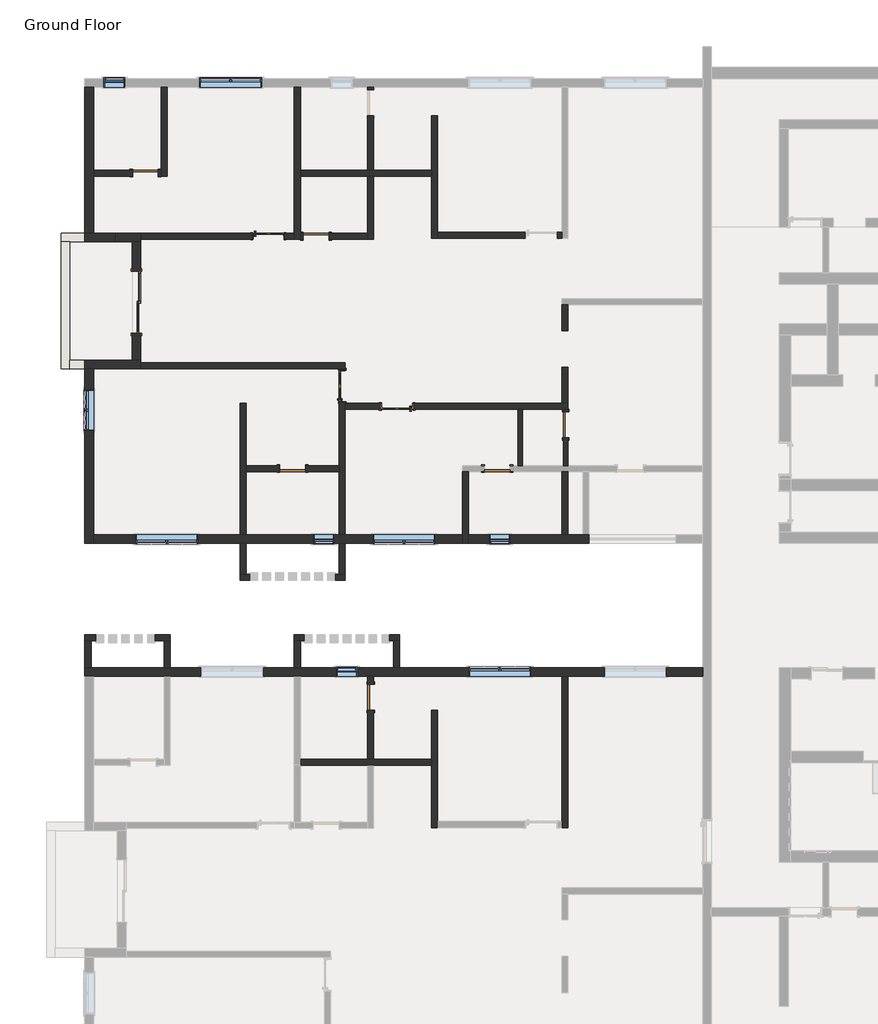
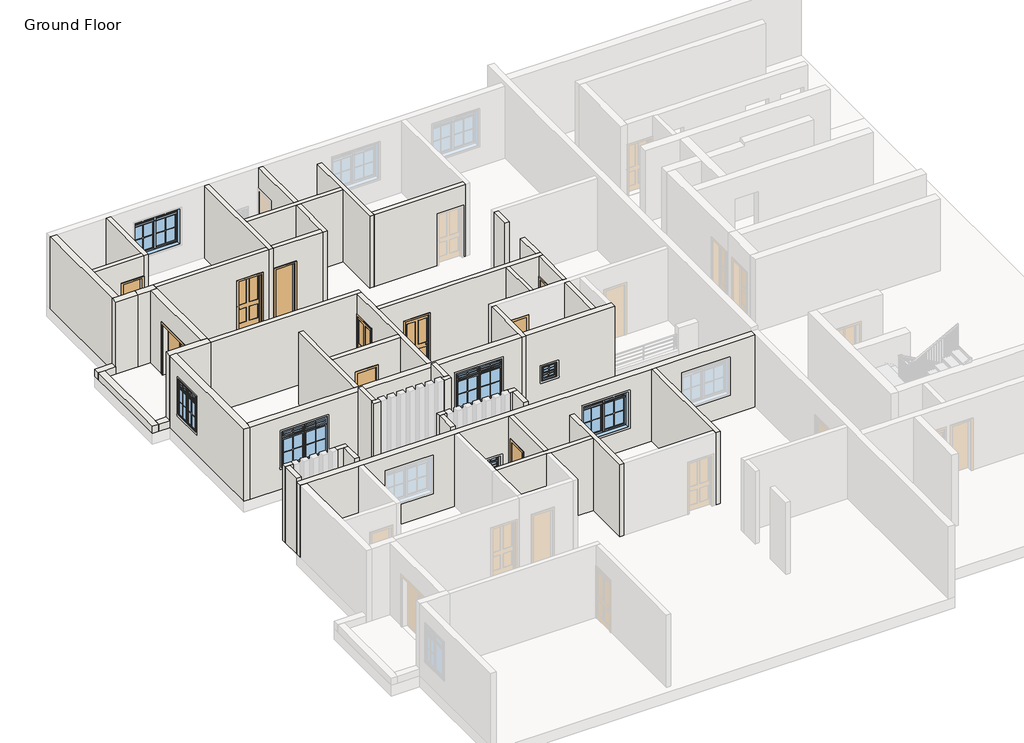
# One storey, part 2 of 9: 49 walls, 10 doors, 9 windows.
"""IFC4 building model written with IfcOpenShell, lengths in millimetres."""

from ifc_helpers import new_model, si_unit, frame, origin, origin_with_axes, place, context, project, spatial, polyline, outline, extrude, faceted_brep, transform, mapped, element, save
from components import door_double_sliding_6_7f701685, door_interior_single_4_panel_wood_3_x_7_bed_room_doors_9f8eaeea, door_0af0cdd0, door_b1104dde, door_6d488673, window_casement_double_awning_double_4_x_5_window_c6f36ef5, window_casement_double_awning_double_6_x_5_2a8633dc, window_double_hung_d0105baa

model = new_model("IFC4")

# Units and contexts
model_context = context("Model", 3, world=origin())
ifc_project = project(units=[si_unit("LENGTHUNIT", "METRE", prefix="MILLI")], contexts=[model_context])

# Site, building, storey
site = spatial("IfcSite", under=ifc_project)
building = spatial("IfcBuilding", under=site)
storey = spatial("IfcBuildingStorey", under=building, Name="Ground Floor", Elevation=0.0)

# Doors
placement = place(None, origin())
door_double_sliding_6_shape = door_double_sliding_6_7f701685(model_context)
element("IfcDoor", 1, ObjectType="Door-Double-Sliding : 6'", at=placement, inside=storey, context=model_context, shape_type="MappedRepresentation", body=[
    mapped(door_double_sliding_6_shape, transform((-13007.9453682, 22386.034892, 0.0), x_axis=(0.0, -1.0, 0.0), y_axis=(1.0, 0.0, 0.0), z_axis=(0.0, 0.0, 1.0))),
])
door_interior_single_4_panel_wood_3_x_7_bed_room_doors_shape = door_interior_single_4_panel_wood_3_x_7_bed_room_doors_9f8eaeea(model_context)
element("IfcDoor", 2, ObjectType="Door-Interior-Single-4_Panel-Wood : 3' x 7' Bed Room Doors", at=placement, inside=storey, context=model_context, shape_type="MappedRepresentation", body=[
    mapped(door_interior_single_4_panel_wood_3_x_7_bed_room_doors_shape, transform((-6826.2203682, 19922.234892, 0.0), x_axis=(0.0, 1.0, 0.0), y_axis=(-1.0, 0.0, 0.0), z_axis=(0.0, 0.0, 1.0))),
])
element("IfcDoor", 3, ObjectType="Door-Interior-Single-4_Panel-Wood : 3' x 7' Bed Room Doors", at=placement, inside=storey, context=model_context, shape_type="MappedRepresentation", body=[
    mapped(door_interior_single_4_panel_wood_3_x_7_bed_room_doors_shape, transform((-5210.1453682, 19322.159892, 0.0), x_axis=(-1.0, 0.0, 0.0), y_axis=(0.0, -1.0, 0.0), z_axis=(0.0, 0.0, 1.0))),
])
element("IfcDoor", 4, ObjectType="Door-Interior-Single-4_Panel-Wood : 3' x 7' Bed Room Doors", at=placement, inside=storey, context=model_context, shape_type="MappedRepresentation", body=[
    mapped(door_interior_single_4_panel_wood_3_x_7_bed_room_doors_shape, transform((-8994.7453682, 24332.309892, 0.0), x_axis=(1.0, 0.0, 0.0), y_axis=(0.0, 1.0, 0.0), z_axis=(0.0, 0.0, 1.0))),
])
door_shape = door_0af0cdd0(model_context)
element("IfcDoor", 5, ObjectType="Single-Flush : 30\" x 80\"", at=placement, inside=storey, context=model_context, shape_type="MappedRepresentation", body=[
    mapped(door_shape, transform((-8283.5453682, 17496.534892, 0.0), x_axis=(-1.0, 0.0, 0.0), y_axis=(0.0, -1.0, 0.0), z_axis=(0.0, 0.0, 1.0))),
])
element("IfcDoor", 6, ObjectType="Single-Flush : 30\" x 80\"", at=placement, inside=storey, context=model_context, shape_type="MappedRepresentation", body=[
    mapped(door_shape, transform((-12614.2453682, 26183.334892, 0.0), x_axis=(1.0, 0.0, 0.0), y_axis=(0.0, 1.0, 0.0), z_axis=(0.0, 0.0, 1.0))),
])
element("IfcDoor", 7, ObjectType="Single-Flush : 30\" x 80\"", at=placement, inside=storey, context=model_context, shape_type="MappedRepresentation", body=[
    mapped(door_shape, transform((-5984.8453682, 10778.234892, 0.0), x_axis=(0.0, 1.0, 0.0), y_axis=(-1.0, 0.0, 0.0), z_axis=(0.0, 0.0, 1.0))),
])
door_2_shape = door_b1104dde(model_context)
element("IfcDoor", 8, ObjectType="Single-Flush : 30\" x 80\"", at=placement, inside=storey, context=model_context, shape_type="MappedRepresentation", body=[
    mapped(door_2_shape, transform((-2263.7453682, 17496.534892, 0.0), x_axis=(1.0, 0.0, 0.0), y_axis=(0.0, 1.0, 0.0), z_axis=(0.0, 0.0, 1.0))),
])
element("IfcDoor", 9, ObjectType="Single-Flush : 30\" x 80\"", at=placement, inside=storey, context=model_context, shape_type="MappedRepresentation", body=[
    mapped(door_2_shape, transform((-7597.7453682, 24329.134892, 0.0), x_axis=(-1.0, 0.0, 0.0), y_axis=(0.0, -1.0, 0.0), z_axis=(0.0, 0.0, 1.0))),
])
door_3_shape = door_6d488673(model_context)
element("IfcDoor", 10, ObjectType="Single-Flush : 30\" x 80\"", at=placement, inside=storey, context=model_context, shape_type="MappedRepresentation", body=[
    mapped(door_3_shape, transform((-250.7953682, 18779.234892, 0.0), x_axis=(0.0, 1.0, 0.0), y_axis=(-1.0, 0.0, 0.0), z_axis=(0.0, 0.0, 1.0))),
])

# Walls
element("IfcWall", 11, at=placement, inside=storey, context=model_context, shape_type="SweptSolid", body=[
    extrude(outline(polyline([(19160.234892, 0.0), (19160.234892, 2133.6), (18398.234892, 2133.6), (18398.234892, 0.0), (17585.434892, 0.0), (17585.434892, 3048.0), (19236.434892, 3048.0), (19236.434892, 0.0), (19160.234892, 0.0)])), frame((-320.6453682, 0.0, 0.0), z_axis=(1.0, 0.0, 0.0), x_axis=(0.0, 1.0, 0.0)), (0.0, 0.0, 1.0), 139.7),
])
element("IfcWall", 12, at=placement, inside=storey, context=model_context, shape_type="SweptSolid", body=[
    extrude(outline(polyline([(-1654.1453682, 17585.434892), (-1654.1453682, 19236.434892), (-1514.4453682, 19236.434892), (-1514.4453682, 17585.434892), (-1654.1453682, 17585.434892)])), origin_with_axes(), (0.0, 0.0, 1.0), 3048.0),
])
element("IfcWall", 13, ObjectType="6\" INTERIOR WALL", at=placement, inside=storey, context=model_context, shape_type="Brep", body=[
    faceted_brep([(-358.7453682, 11387.834892, 0.0), (-358.7453682, 7120.634892, 0.0), (-358.7453682, 6942.834892, 0.0), (-358.7453682, 6942.834892, 3048.0), (-358.7453682, 11387.834892, 3048.0), (-180.9453682, 6942.834892, 0.0), (-180.9453682, 11387.834892, 0.0), (-180.9453682, 11387.834892, 3048.0), (-180.9453682, 6942.834892, 3048.0)], [[[0, 1, 2, 3, 4]], [[5, 6, 7, 8]], [[2, 1, 0, 6, 5]], [[6, 0, 4, 7]], [[2, 5, 8, 3]], [[4, 3, 8, 7]]]),
])
element("IfcWall", 14, ObjectType="6\" INTERIOR WALL", at=placement, inside=storey, context=model_context, shape_type="Brep", body=[
    faceted_brep([(-4194.1453682, 10397.234892, 0.0), (-4194.1453682, 8949.434892, 0.0), (-4194.1453682, 8771.634892, 0.0), (-4194.1453682, 6942.834892, 0.0), (-4194.1453682, 6942.834892, 3048.0), (-4194.1453682, 8771.634892, 3048.0), (-4194.1453682, 8949.434892, 3048.0), (-4194.1453682, 10397.234892, 3048.0), (-4016.3453682, 6942.834892, 0.0), (-4016.3453682, 7120.634892, 0.0), (-4016.3453682, 10397.234892, 0.0), (-4016.3453682, 10397.234892, 3048.0), (-4016.3453682, 7120.634892, 3048.0), (-4016.3453682, 6942.834892, 3048.0)], [[[0, 1, 2, 3, 4, 5, 6, 7]], [[8, 9, 10, 11, 12, 13]], [[3, 2, 1, 0, 10, 9, 8]], [[10, 0, 7, 11]], [[3, 8, 13, 4]], [[7, 6, 5, 4, 13, 12, 11]]]),
])
element("IfcWall", 15, ObjectType="6\" INTERIOR WALL", at=placement, inside=storey, context=model_context, shape_type="SweptSolid", body=[
    extrude(outline(polyline([(11159.234892, 0.0), (11159.234892, 2133.6), (10397.234892, 2133.6), (10397.234892, 0.0), (8949.434892, 0.0), (8949.434892, 3048.0), (11387.834892, 3048.0), (11387.834892, 0.0), (11159.234892, 0.0)])), frame((-6073.7453682, 0.0, 0.0), z_axis=(1.0, 0.0, 0.0), x_axis=(0.0, 1.0, 0.0)), (0.0, 0.0, 1.0), 177.8),
])
element("IfcWall", 16, ObjectType="6\" INTERIOR WALL", at=placement, inside=storey, context=model_context, shape_type="Brep", body=[
    faceted_brep([(-8054.9453682, 8771.634892, 0.0), (-6073.7453682, 8771.634892, 0.0), (-5895.9453682, 8771.634892, 0.0), (-4194.1453682, 8771.634892, 0.0), (-4194.1453682, 8771.634892, 3048.0), (-5895.9453682, 8771.634892, 3048.0), (-6073.7453682, 8771.634892, 3048.0), (-8054.9453682, 8771.634892, 3048.0), (-4194.1453682, 8949.434892, 0.0), (-5895.9453682, 8949.434892, 0.0), (-6073.7453682, 8949.434892, 0.0), (-8054.9453682, 8949.434892, 0.0), (-8054.9453682, 8949.434892, 3048.0), (-6073.7453682, 8949.434892, 3048.0), (-5895.9453682, 8949.434892, 3048.0), (-4194.1453682, 8949.434892, 3048.0)], [[[0, 1, 2, 3, 4, 5, 6, 7]], [[8, 9, 10, 11, 12, 13, 14, 15]], [[3, 2, 1, 0, 11, 10, 9, 8]], [[11, 0, 7, 12]], [[3, 8, 15, 4]], [[7, 6, 5, 4, 15, 14, 13, 12]]]),
])
element("IfcWall", 17, ObjectType="6\" INTERIOR WALL", at=placement, inside=storey, context=model_context, shape_type="SweptSolid", body=[
    extrude(outline(polyline([(-358.7453682, 15553.434892), (-358.7453682, 17407.634892), (-180.9453682, 17407.634892), (-180.9453682, 15553.434892), (-358.7453682, 15553.434892)])), origin_with_axes(), (0.0, 0.0, 1.0), 3048.0),
])
element("IfcWall", 18, ObjectType="6\" INTERIOR WALL", at=placement, inside=storey, context=model_context, shape_type="Brep", body=[
    faceted_brep([(-5692.7453682, 19414.234892, 0.0), (-6734.1453682, 19414.234892, 0.0), (-6734.1453682, 19414.234892, 3048.0), (-358.7453682, 19414.234892, 3048.0), (-180.9453682, 19414.234892, 3048.0), (-180.9453682, 19414.234892, 0.0), (-358.7453682, 19414.234892, 0.0), (-4727.5453682, 19414.234892, 0.0), (-4727.5453682, 19414.234892, 2159.0), (-5692.7453682, 19414.234892, 2159.0), (-6734.1453682, 19236.434892, 0.0), (-5692.7453682, 19236.434892, 0.0), (-5692.7453682, 19236.434892, 2159.0), (-4727.5453682, 19236.434892, 2159.0), (-4727.5453682, 19236.434892, 0.0), (-1654.1453682, 19236.434892, 0.0), (-1514.4453682, 19236.434892, 0.0), (-320.6453682, 19236.434892, 0.0), (-180.9453682, 19236.434892, 0.0), (-180.9453682, 19236.434892, 3048.0), (-320.6453682, 19236.434892, 3048.0), (-1514.4453682, 19236.434892, 3048.0), (-1654.1453682, 19236.434892, 3048.0), (-6734.1453682, 19236.434892, 3048.0)], [[[0, 1, 2, 3, 4, 5, 6, 7, 8, 9]], [[10, 11, 12, 13, 14, 15, 16, 17, 18, 19, 20, 21, 22, 23]], [[5, 18, 17, 16, 15, 14, 7, 6]], [[10, 1, 0, 11]], [[18, 5, 4, 19]], [[1, 10, 23, 2]], [[4, 3, 2, 23, 22, 21, 20, 19]], [[9, 12, 11, 0]], [[12, 9, 8, 13]], [[13, 8, 7, 14]]]),
])
element("IfcWall", 19, ObjectType="6\" INTERIOR WALL", at=placement, inside=storey, context=model_context, shape_type="Brep", body=[
    faceted_brep([(-3279.7453682, 17407.634892, 0.0), (-3279.7453682, 15553.434892, 0.0), (-3279.7453682, 15299.434892, 0.0), (-3279.7453682, 15299.434892, 3048.0), (-3279.7453682, 15553.434892, 3048.0), (-3279.7453682, 17407.634892, 3048.0), (-3101.9453682, 15299.434892, 0.0), (-3101.9453682, 15553.434892, 0.0), (-3101.9453682, 17407.634892, 0.0), (-3101.9453682, 17407.634892, 3048.0), (-3101.9453682, 15299.434892, 3048.0)], [[[0, 1, 2, 3, 4, 5]], [[6, 7, 8, 9, 10]], [[2, 1, 0, 8, 7, 6]], [[8, 0, 5, 9]], [[2, 6, 10, 3]], [[5, 4, 3, 10, 9]]]),
])
element("IfcWall", 20, ObjectType="6\" INTERIOR WALL", at=placement, inside=storey, context=model_context, shape_type="Brep", body=[
    faceted_brep([(-9655.1453682, 15553.434892, 0.0), (-9655.1453682, 17407.634892, 0.0), (-9655.1453682, 17585.434892, 0.0), (-9655.1453682, 19414.234892, 0.0), (-9655.1453682, 19414.234892, 3048.0), (-9655.1453682, 17585.434892, 3048.0), (-9655.1453682, 17407.634892, 3048.0), (-9655.1453682, 15553.434892, 3048.0), (-9832.9453682, 19414.234892, 0.0), (-9832.9453682, 15553.434892, 0.0), (-9832.9453682, 15553.434892, 3048.0), (-9832.9453682, 19414.234892, 3048.0)], [[[0, 1, 2, 3, 4, 5, 6, 7]], [[8, 9, 10, 11]], [[3, 2, 1, 0, 9, 8]], [[3, 8, 11, 4]], [[9, 0, 7, 10]], [[7, 6, 5, 4, 11, 10]]]),
])
element("IfcWall", 21, ObjectType="6\" INTERIOR WALL", at=placement, inside=storey, context=model_context, shape_type="SweptSolid", body=[
    extrude(outline(polyline([(0.0, -8664.5453682), (2133.6, -8664.5453682), (2133.6, -7902.5453682), (0.0, -7902.5453682), (0.0, -6911.9453682), (3048.0, -6911.9453682), (3048.0, -9655.1453682), (0.0, -9655.1453682), (0.0, -8664.5453682)])), frame((0.0, 17407.634892, 0.0), z_axis=(0.0, 1.0, 0.0), x_axis=(0.0, 0.0, 1.0)), (0.0, 0.0, 1.0), 177.8),
])
element("IfcWall", 22, ObjectType="6\" INTERIOR WALL", at=placement, inside=storey, context=model_context, shape_type="Brep", body=[
    faceted_brep([(-6911.9453682, 20430.234892, 0.0), (-6911.9453682, 20404.834892, 0.0), (-6911.9453682, 20404.834892, 2159.0), (-6911.9453682, 19439.634892, 2159.0), (-6911.9453682, 19439.634892, 0.0), (-6911.9453682, 17585.434892, 0.0), (-6911.9453682, 17407.634892, 0.0), (-6911.9453682, 15553.434892, 0.0), (-6911.9453682, 15553.434892, 3048.0), (-6911.9453682, 17407.634892, 3048.0), (-6911.9453682, 17585.434892, 3048.0), (-6911.9453682, 20430.234892, 3048.0), (-6734.1453682, 20404.834892, 0.0), (-6734.1453682, 20430.234892, 0.0), (-6734.1453682, 20430.234892, 3048.0), (-6734.1453682, 19414.234892, 3048.0), (-6734.1453682, 19236.434892, 3048.0), (-6734.1453682, 15553.434892, 3048.0), (-6734.1453682, 15553.434892, 0.0), (-6734.1453682, 19236.434892, 0.0), (-6734.1453682, 19414.234892, 0.0), (-6734.1453682, 19439.634892, 0.0), (-6734.1453682, 19439.634892, 2159.0), (-6734.1453682, 20404.834892, 2159.0)], [[[0, 1, 2, 3, 4, 5, 6, 7, 8, 9, 10, 11]], [[12, 13, 14, 15, 16, 17, 18, 19, 20, 21, 22, 23]], [[18, 7, 6, 5, 4, 21, 20, 19]], [[0, 13, 12, 1]], [[7, 18, 17, 8]], [[13, 0, 11, 14]], [[11, 10, 9, 8, 17, 16, 15, 14]], [[23, 2, 1, 12]], [[2, 23, 22, 3]], [[3, 22, 21, 4]]]),
])
element("IfcWall", 23, ObjectType="6\" INTERIOR WALL", at=placement, inside=storey, context=model_context, shape_type="SweptSolid", body=[
    extrude(outline(polyline([(-358.7453682, 21547.834892), (-358.7453682, 22309.834892), (-180.9453682, 22309.834892), (-180.9453682, 21547.834892), (-358.7453682, 21547.834892)])), origin_with_axes(), (0.0, 0.0, 1.0), 3048.0),
])
element("IfcWall", 24, ObjectType="6\" INTERIOR WALL", at=placement, inside=storey, context=model_context, shape_type="SweptSolid", body=[
    extrude(outline(polyline([(-358.7453682, 19414.234892), (-358.7453682, 20481.034892), (-180.9453682, 20481.034892), (-180.9453682, 19414.234892), (-358.7453682, 19414.234892)])), origin_with_axes(), (0.0, 0.0, 1.0), 3048.0),
])
element("IfcWall", 25, ObjectType="6\" INTERIOR WALL", at=placement, inside=storey, context=model_context, shape_type="Brep", body=[
    faceted_brep([(-4194.1453682, 27872.434892, 0.0), (-4194.1453682, 26272.234892, 0.0), (-4194.1453682, 26094.434892, 0.0), (-4194.1453682, 24265.634892, 0.0), (-4194.1453682, 24265.634892, 3048.0), (-4194.1453682, 26094.434892, 3048.0), (-4194.1453682, 26272.234892, 3048.0), (-4194.1453682, 27872.434892, 3048.0), (-4016.3453682, 24265.634892, 0.0), (-4016.3453682, 24443.434892, 0.0), (-4016.3453682, 27872.434892, 0.0), (-4016.3453682, 27872.434892, 3048.0), (-4016.3453682, 24443.434892, 3048.0), (-4016.3453682, 24265.634892, 3048.0)], [[[0, 1, 2, 3, 4, 5, 6, 7]], [[8, 9, 10, 11, 12, 13]], [[3, 2, 1, 0, 10, 9, 8]], [[10, 0, 7, 11]], [[3, 8, 13, 4]], [[7, 6, 5, 4, 13, 12, 11]]]),
])
element("IfcWall", 26, ObjectType="6\" INTERIOR WALL", at=placement, inside=storey, context=model_context, shape_type="SweptSolid", body=[
    extrude(outline(polyline([(28634.434892, 0.0), (28634.434892, 2133.6), (27872.434892, 2133.6), (27872.434892, 0.0), (26272.234892, 0.0), (26272.234892, 3048.0), (28710.634892, 3048.0), (28710.634892, 0.0), (28634.434892, 0.0)])), frame((-6073.7453682, 0.0, 0.0), z_axis=(1.0, 0.0, 0.0), x_axis=(0.0, 1.0, 0.0)), (0.0, 0.0, 1.0), 177.8),
])
element("IfcWall", 27, ObjectType="6\" INTERIOR WALL", at=placement, inside=storey, context=model_context, shape_type="Brep", body=[
    faceted_brep([(-8054.9453682, 26094.434892, 0.0), (-6073.7453682, 26094.434892, 0.0), (-5895.9453682, 26094.434892, 0.0), (-4194.1453682, 26094.434892, 0.0), (-4194.1453682, 26094.434892, 3048.0), (-5895.9453682, 26094.434892, 3048.0), (-6073.7453682, 26094.434892, 3048.0), (-8054.9453682, 26094.434892, 3048.0), (-4194.1453682, 26272.234892, 0.0), (-5895.9453682, 26272.234892, 0.0), (-6073.7453682, 26272.234892, 0.0), (-8054.9453682, 26272.234892, 0.0), (-8054.9453682, 26272.234892, 3048.0), (-6073.7453682, 26272.234892, 3048.0), (-5895.9453682, 26272.234892, 3048.0), (-4194.1453682, 26272.234892, 3048.0)], [[[0, 1, 2, 3, 4, 5, 6, 7]], [[8, 9, 10, 11, 12, 13, 14, 15]], [[3, 2, 1, 0, 11, 10, 9, 8]], [[3, 8, 15, 4]], [[11, 0, 7, 12]], [[7, 6, 5, 4, 15, 14, 13, 12]]]),
])
element("IfcWall", 28, ObjectType="6\" INTERIOR WALL", at=placement, inside=storey, context=model_context, shape_type="Brep", body=[
    faceted_brep([(-8232.7453682, 28710.634892, 0.0), (-8232.7453682, 24418.034892, 0.0), (-8232.7453682, 24240.234892, 0.0), (-8232.7453682, 24240.234892, 3048.0), (-8232.7453682, 28710.634892, 3048.0), (-8054.9453682, 24240.234892, 0.0), (-8054.9453682, 24418.034892, 0.0), (-8054.9453682, 26094.434892, 0.0), (-8054.9453682, 26272.234892, 0.0), (-8054.9453682, 28710.634892, 0.0), (-8054.9453682, 28710.634892, 3048.0), (-8054.9453682, 26272.234892, 3048.0), (-8054.9453682, 26094.434892, 3048.0), (-8054.9453682, 24418.034892, 3048.0), (-8054.9453682, 24240.234892, 3048.0)], [[[0, 1, 2, 3, 4]], [[5, 6, 7, 8, 9, 10, 11, 12, 13, 14]], [[2, 1, 0, 9, 8, 7, 6, 5]], [[9, 0, 4, 10]], [[2, 5, 14, 3]], [[4, 3, 14, 13, 12, 11, 10]]]),
])
element("IfcWall", 29, ObjectType="6\" INTERIOR WALL", at=placement, inside=storey, context=model_context, shape_type="Brep", body=[
    faceted_brep([(-12157.0453682, 28710.634892, 0.0), (-12157.0453682, 26272.234892, 0.0), (-12157.0453682, 26094.434892, 0.0), (-12157.0453682, 26094.434892, 3048.0), (-12157.0453682, 28710.634892, 3048.0), (-11979.2453682, 26094.434892, 0.0), (-11979.2453682, 28710.634892, 0.0), (-11979.2453682, 28710.634892, 3048.0), (-11979.2453682, 26094.434892, 3048.0)], [[[0, 1, 2, 3, 4]], [[5, 6, 7, 8]], [[2, 1, 0, 6, 5]], [[6, 0, 4, 7]], [[2, 5, 8, 3]], [[4, 3, 8, 7]]]),
])
element("IfcWall", 30, ObjectType="6\" INTERIOR WALL", at=placement, inside=storey, context=model_context, shape_type="SweptSolid", body=[
    extrude(outline(polyline([(2133.6, -12233.2453682), (0.0, -12233.2453682), (0.0, -12157.0453682), (3048.0, -12157.0453682), (3048.0, -14138.2453682), (0.0, -14138.2453682), (0.0, -12995.2453682), (2133.6, -12995.2453682), (2133.6, -12233.2453682)])), frame((0.0, 26094.434892, 0.0), z_axis=(0.0, 1.0, 0.0), x_axis=(0.0, 0.0, 1.0)), (0.0, 0.0, 1.0), 177.8),
])
element("IfcWall", 31, ObjectType="6\" INTERIOR WALL", at=placement, inside=storey, context=model_context, shape_type="Brep", body=[
    faceted_brep([(-6073.7453682, 26094.434892, 0.0), (-6073.7453682, 24418.034892, 0.0), (-6073.7453682, 24240.234892, 0.0), (-6073.7453682, 24240.234892, 3048.0), (-6073.7453682, 26094.434892, 3048.0), (-5895.9453682, 24240.234892, 0.0), (-5895.9453682, 26094.434892, 0.0), (-5895.9453682, 26094.434892, 3048.0), (-5895.9453682, 24240.234892, 3048.0)], [[[0, 1, 2, 3, 4]], [[5, 6, 7, 8]], [[2, 1, 0, 6, 5]], [[6, 0, 4, 7]], [[2, 5, 8, 3]], [[4, 3, 8, 7]]]),
])
element("IfcWall", 32, ObjectType="6\" INTERIOR WALL", at=placement, inside=storey, context=model_context, shape_type="SweptSolid", body=[
    extrude(outline(polyline([(0.0, -7978.7453682), (2133.6, -7978.7453682), (2133.6, -7216.7453682), (0.0, -7216.7453682), (0.0, -6073.7453682), (3048.0, -6073.7453682), (3048.0, -8054.9453682), (0.0, -8054.9453682), (0.0, -7978.7453682)])), frame((0.0, 24240.234892, 0.0), z_axis=(0.0, 1.0, 0.0), x_axis=(0.0, 0.0, 1.0)), (0.0, 0.0, 1.0), 177.8),
])
element("IfcWall", 33, ObjectType="6\" INTERIOR WALL", at=placement, inside=storey, context=model_context, shape_type="SweptSolid", body=[
    extrude(outline(polyline([(0.0, -485.7453682), (0.0, -358.7453682), (3048.0, -358.7453682), (3048.0, -4016.3453682), (0.0, -4016.3453682), (0.0, -1450.9453682), (2159.0, -1450.9453682), (2159.0, -485.7453682), (0.0, -485.7453682)])), frame((0.0, 24265.634892, 0.0), z_axis=(0.0, 1.0, 0.0), x_axis=(0.0, 0.0, 1.0)), (0.0, 0.0, 1.0), 177.8),
])
element("IfcWall", 34, ObjectType="6\" INTERIOR WALL", at=placement, inside=storey, context=model_context, shape_type="Brep", body=[
    faceted_brep([(-12753.9453682, 20430.234892, 0.0), (-6911.9453682, 20430.234892, 0.0), (-6734.1453682, 20430.234892, 0.0), (-6734.1453682, 20430.234892, 3048.0), (-12753.9453682, 20430.234892, 3048.0), (-6734.1453682, 20608.034892, 0.0), (-12753.9453682, 20608.034892, 0.0), (-12753.9453682, 20608.034892, 3048.0), (-6734.1453682, 20608.034892, 3048.0)], [[[0, 1, 2, 3, 4]], [[5, 6, 7, 8]], [[2, 1, 0, 6, 5]], [[6, 0, 4, 7]], [[2, 5, 8, 3]], [[4, 3, 8, 7]]]),
])
element("IfcWall", 35, ObjectType="6\" INTERIOR WALL", at=placement, inside=storey, context=model_context, shape_type="SweptSolid", body=[
    extrude(outline(polyline([(0.0, -8512.1453682), (0.0, -8232.7453682), (3048.0, -8232.7453682), (3048.0, -12753.9453682), (0.0, -12753.9453682), (0.0, -9477.3453682), (2159.0, -9477.3453682), (2159.0, -8512.1453682), (0.0, -8512.1453682)])), frame((0.0, 24240.234892, 0.0), z_axis=(0.0, 1.0, 0.0), x_axis=(0.0, 0.0, 1.0)), (0.0, 0.0, 1.0), 177.8),
])
element("IfcWall", 36, ObjectType="6\" INTERIOR WALL", at=placement, inside=storey, context=model_context, shape_type="SweptSolid", body=[
    extrude(outline(polyline([(-8054.9453682, 12429.234892), (-8054.9453682, 11641.834892), (-8232.7453682, 11641.834892), (-8232.7453682, 12429.234892), (-8054.9453682, 12429.234892)])), origin_with_axes(), (0.0, 0.0, 1.0), 3200.4),
])
element("IfcWall", 37, ObjectType="6\" INTERIOR WALL", at=placement, inside=storey, context=model_context, shape_type="SweptSolid", body=[
    extrude(outline(polyline([(-5133.9453682, 12429.234892), (-5133.9453682, 11641.834892), (-5311.7453682, 11641.834892), (-5311.7453682, 12429.234892), (-5133.9453682, 12429.234892)])), origin_with_axes(), (0.0, 0.0, 1.0), 3200.4),
])
element("IfcWall", 38, ObjectType="6\" INTERIOR WALL", at=placement, inside=storey, context=model_context, shape_type="Brep", body=[
    faceted_brep([(-8232.7453682, 12429.234892, 0.0), (-8054.9453682, 12429.234892, 0.0), (-7940.6453682, 12429.234892, 0.0), (-7940.6453682, 12429.234892, 3200.4), (-8054.9453682, 12429.234892, 3200.4), (-8232.7453682, 12429.234892, 3200.4), (-8232.7453682, 12607.034892, 0.0), (-8232.7453682, 12607.034892, 3200.4), (-7940.6453682, 12607.034892, 3200.4), (-7940.6453682, 12607.034892, 0.0)], [[[0, 1, 2, 3, 4, 5]], [[6, 7, 8, 9]], [[2, 1, 0, 6, 9]], [[3, 2, 9, 8]], [[5, 4, 3, 8, 7]], [[0, 5, 7, 6]]]),
])
element("IfcWall", 39, ObjectType="6\" INTERIOR WALL", at=placement, inside=storey, context=model_context, shape_type="Brep", body=[
    faceted_brep([(-5133.9453682, 12607.034892, 0.0), (-5426.0453682, 12607.034892, 0.0), (-5426.0453682, 12607.034892, 3200.4), (-5133.9453682, 12607.034892, 3200.4), (-5133.9453682, 12429.234892, 0.0), (-5133.9453682, 12429.234892, 3200.4), (-5311.7453682, 12429.234892, 3200.4), (-5426.0453682, 12429.234892, 3200.4), (-5426.0453682, 12429.234892, 0.0), (-5311.7453682, 12429.234892, 0.0)], [[[0, 1, 2, 3]], [[4, 5, 6, 7, 8, 9]], [[1, 0, 4, 9, 8]], [[2, 1, 8, 7]], [[3, 2, 7, 6, 5]], [[0, 3, 5, 4]]]),
])
element("IfcWall", 40, ObjectType="6\" INTERIOR WALL", at=placement, inside=storey, context=model_context, shape_type="Brep", body=[
    faceted_brep([(-14214.4453682, 11641.834892, 0.0), (-14214.4453682, 12429.234892, 0.0), (-14214.4453682, 12429.234892, 3200.4), (-14214.4453682, 11641.834892, 3200.4), (-14392.2453682, 11641.834892, 0.0), (-14392.2453682, 11641.834892, 3048.0), (-14392.2453682, 11641.834892, 3200.4), (-14392.2453682, 12429.234892, 3200.4), (-14392.2453682, 12429.234892, 0.0)], [[[0, 1, 2, 3]], [[4, 5, 6, 7, 8]], [[1, 0, 4, 8]], [[3, 2, 7, 6]], [[2, 1, 8, 7]], [[0, 3, 6, 5, 4]]]),
])
element("IfcWall", 41, ObjectType="6\" INTERIOR WALL", at=placement, inside=storey, context=model_context, shape_type="SweptSolid", body=[
    extrude(outline(polyline([(-11890.3453682, 12429.234892), (-11890.3453682, 11641.834892), (-12068.1453682, 11641.834892), (-12068.1453682, 12429.234892), (-11890.3453682, 12429.234892)])), origin_with_axes(), (0.0, 0.0, 1.0), 3200.4),
])
element("IfcWall", 42, ObjectType="6\" INTERIOR WALL", at=placement, inside=storey, context=model_context, shape_type="Brep", body=[
    faceted_brep([(-14392.2453682, 12429.234892, 0.0), (-14214.4453682, 12429.234892, 0.0), (-14074.7453682, 12429.234892, 0.0), (-14074.7453682, 12429.234892, 3200.4), (-14214.4453682, 12429.234892, 3200.4), (-14392.2453682, 12429.234892, 3200.4), (-14392.2453682, 12607.034892, 0.0), (-14392.2453682, 12607.034892, 3200.4), (-14074.7453682, 12607.034892, 3200.4), (-14074.7453682, 12607.034892, 0.0)], [[[0, 1, 2, 3, 4, 5]], [[6, 7, 8, 9]], [[2, 1, 0, 6, 9]], [[3, 2, 9, 8]], [[5, 4, 3, 8, 7]], [[0, 5, 7, 6]]]),
])
element("IfcWall", 43, ObjectType="6\" INTERIOR WALL", at=placement, inside=storey, context=model_context, shape_type="Brep", body=[
    faceted_brep([(-11890.3453682, 12607.034892, 0.0), (-12322.1453682, 12607.034892, 0.0), (-12322.1453682, 12607.034892, 3200.4), (-11890.3453682, 12607.034892, 3200.4), (-11890.3453682, 12429.234892, 0.0), (-11890.3453682, 12429.234892, 3200.4), (-12068.1453682, 12429.234892, 3200.4), (-12322.1453682, 12429.234892, 3200.4), (-12322.1453682, 12429.234892, 0.0), (-12068.1453682, 12429.234892, 0.0)], [[[0, 1, 2, 3]], [[4, 5, 6, 7, 8, 9]], [[1, 0, 4, 9, 8]], [[2, 1, 8, 7]], [[3, 2, 7, 6, 5]], [[0, 3, 5, 4]]]),
])
element("IfcWall", 44, ObjectType="6\" INTERIOR WALL", at=placement, inside=storey, context=model_context, shape_type="SweptSolid", body=[
    extrude(outline(polyline([(-9832.9453682, 14385.034892), (-9832.9453682, 15299.434892), (-9655.1453682, 15299.434892), (-9655.1453682, 14385.034892), (-9832.9453682, 14385.034892)])), origin_with_axes(), (0.0, 0.0, 1.0), 3200.4),
])
element("IfcWall", 45, ObjectType="6\" INTERIOR WALL", at=placement, inside=storey, context=model_context, shape_type="SweptSolid", body=[
    extrude(outline(polyline([(-6911.9453682, 14385.034892), (-6911.9453682, 15299.434892), (-6734.1453682, 15299.434892), (-6734.1453682, 14385.034892), (-6911.9453682, 14385.034892)])), origin_with_axes(), (0.0, 0.0, 1.0), 3200.4),
])
element("IfcWall", 46, ObjectType="6\" INTERIOR WALL", at=placement, inside=storey, context=model_context, shape_type="Brep", body=[
    faceted_brep([(-9832.9453682, 14207.234892, 0.0), (-9540.8453682, 14207.234892, 0.0), (-9540.8453682, 14207.234892, 3200.4), (-9832.9453682, 14207.234892, 3200.4), (-9832.9453682, 14385.034892, 0.0), (-9832.9453682, 14385.034892, 3200.4), (-9655.1453682, 14385.034892, 3200.4), (-9540.8453682, 14385.034892, 3200.4), (-9540.8453682, 14385.034892, 0.0), (-9655.1453682, 14385.034892, 0.0)], [[[0, 1, 2, 3]], [[4, 5, 6, 7, 8, 9]], [[1, 0, 4, 9, 8]], [[2, 1, 8, 7]], [[3, 2, 7, 6, 5]], [[0, 3, 5, 4]]]),
])
element("IfcWall", 47, ObjectType="6\" INTERIOR WALL", at=placement, inside=storey, context=model_context, shape_type="Brep", body=[
    faceted_brep([(-6734.1453682, 14385.034892, 0.0), (-6911.9453682, 14385.034892, 0.0), (-7026.2453682, 14385.034892, 0.0), (-7026.2453682, 14385.034892, 3200.4), (-6911.9453682, 14385.034892, 3200.4), (-6734.1453682, 14385.034892, 3200.4), (-6734.1453682, 14207.234892, 0.0), (-6734.1453682, 14207.234892, 3200.4), (-7026.2453682, 14207.234892, 3200.4), (-7026.2453682, 14207.234892, 0.0)], [[[0, 1, 2, 3, 4, 5]], [[6, 7, 8, 9]], [[2, 1, 0, 6, 9]], [[3, 2, 9, 8]], [[5, 4, 3, 8, 7]], [[0, 5, 7, 6]]]),
])
element("IfcWall", 48, ObjectType="9\" EXTERIOR WALL", at=placement, inside=storey, context=model_context, shape_type="Brep", body=[
    faceted_brep([(3781.4546318, 11641.834892, 0.0), (-5133.9453682, 11641.834892, 0.0), (-5311.7453682, 11641.834892, 0.0), (-8054.9453682, 11641.834892, 0.0), (-8232.7453682, 11641.834892, 0.0), (-11890.3453682, 11641.834892, 0.0), (-12068.1453682, 11641.834892, 0.0), (-14214.4453682, 11641.834892, 0.0), (-14392.2453682, 11641.834892, 0.0), (-14392.2453682, 11641.834892, 3048.0), (3781.4546318, 11641.834892, 3048.0), (-9147.1453682, 11641.834892, 914.4), (-9147.1453682, 11641.834892, 2438.4), (-10975.9453682, 11641.834892, 2438.4), (-10975.9453682, 11641.834892, 914.4), (-1273.1453682, 11641.834892, 914.4), (-1273.1453682, 11641.834892, 2438.4), (-3101.9453682, 11641.834892, 2438.4), (-3101.9453682, 11641.834892, 914.4), (2714.6546318, 11641.834892, 914.4), (2714.6546318, 11641.834892, 2438.4), (885.8546318, 11641.834892, 2438.4), (885.8546318, 11641.834892, 914.4), (-6988.1453682, 11641.834892, 1524.0), (-6988.1453682, 11641.834892, 914.4), (-6378.5453682, 11641.834892, 914.4), (-6378.5453682, 11641.834892, 1524.0), (-14392.2453682, 11387.834892, 0.0), (-14138.2453682, 11387.834892, 0.0), (-12068.1453682, 11387.834892, 0.0), (-11890.3453682, 11387.834892, 0.0), (-8232.7453682, 11387.834892, 0.0), (-8054.9453682, 11387.834892, 0.0), (-6073.7453682, 11387.834892, 0.0), (-5895.9453682, 11387.834892, 0.0), (-358.7453682, 11387.834892, 0.0), (-180.9453682, 11387.834892, 0.0), (3781.4546318, 11387.834892, 0.0), (3781.4546318, 11387.834892, 3048.0), (-180.9453682, 11387.834892, 3048.0), (-358.7453682, 11387.834892, 3048.0), (-5895.9453682, 11387.834892, 3048.0), (-6073.7453682, 11387.834892, 3048.0), (-8054.9453682, 11387.834892, 3048.0), (-8232.7453682, 11387.834892, 3048.0), (-11890.3453682, 11387.834892, 3048.0), (-12068.1453682, 11387.834892, 3048.0), (-14138.2453682, 11387.834892, 3048.0), (-14392.2453682, 11387.834892, 3048.0), (-9147.1453682, 11387.834892, 2438.4), (-9147.1453682, 11387.834892, 914.4), (-10975.9453682, 11387.834892, 914.4), (-10975.9453682, 11387.834892, 2438.4), (-1273.1453682, 11387.834892, 2438.4), (-1273.1453682, 11387.834892, 914.4), (-3101.9453682, 11387.834892, 914.4), (-3101.9453682, 11387.834892, 2438.4), (2714.6546318, 11387.834892, 2438.4), (2714.6546318, 11387.834892, 914.4), (885.8546318, 11387.834892, 914.4), (885.8546318, 11387.834892, 2438.4), (-6988.1453682, 11387.834892, 914.4), (-6988.1453682, 11387.834892, 1524.0), (-6378.5453682, 11387.834892, 1524.0), (-6378.5453682, 11387.834892, 914.4)], [[[0, 1, 2, 3, 4, 5, 6, 7, 8, 9, 10], [11, 12, 13, 14], [15, 16, 17, 18], [19, 20, 21, 22], [23, 24, 25, 26]], [[27, 28, 29, 30, 31, 32, 33, 34, 35, 36, 37, 38, 39, 40, 41, 42, 43, 44, 45, 46, 47, 48], [49, 50, 51, 52], [53, 54, 55, 56], [57, 58, 59, 60], [61, 62, 63, 64]], [[8, 7, 6, 5, 4, 3, 2, 1, 0, 37, 36, 35, 34, 33, 32, 31, 30, 29, 28, 27]], [[37, 0, 10, 38]], [[8, 27, 48, 9]], [[10, 9, 48, 47, 46, 45, 44, 43, 42, 41, 40, 39, 38]], [[50, 49, 12, 11]], [[51, 50, 11, 14]], [[52, 51, 14, 13]], [[49, 52, 13, 12]], [[54, 53, 16, 15]], [[55, 54, 15, 18]], [[56, 55, 18, 17]], [[53, 56, 17, 16]], [[58, 57, 20, 19]], [[59, 58, 19, 22]], [[60, 59, 22, 21]], [[57, 60, 21, 20]], [[24, 23, 62, 61]], [[25, 24, 61, 64]], [[26, 25, 64, 63]], [[23, 26, 63, 62]]]),
])
element("IfcWall", 49, ObjectType="9\" EXTERIOR WALL", at=placement, inside=storey, context=model_context, shape_type="Brep", body=[
    faceted_brep([(-14138.2453682, 15299.434892, 0.0), (-14138.2453682, 15553.434892, 0.0), (-14138.2453682, 20430.234892, 0.0), (-14138.2453682, 20430.234892, 3048.0), (-14138.2453682, 15553.434892, 3048.0), (-14138.2453682, 15299.434892, 3048.0), (-14138.2453682, 19820.634892, 2438.4), (-14138.2453682, 19820.634892, 914.4), (-14138.2453682, 18601.434892, 914.4), (-14138.2453682, 18601.434892, 2438.4), (-14392.2453682, 20430.234892, 0.0), (-14392.2453682, 15299.434892, 0.0), (-14392.2453682, 15299.434892, 3048.0), (-14392.2453682, 20430.234892, 3048.0), (-14392.2453682, 19820.634892, 914.4), (-14392.2453682, 19820.634892, 2438.4), (-14392.2453682, 18601.434892, 2438.4), (-14392.2453682, 18601.434892, 914.4)], [[[0, 1, 2, 3, 4, 5], [6, 7, 8, 9]], [[10, 11, 12, 13], [14, 15, 16, 17]], [[2, 1, 0, 11, 10]], [[11, 0, 5, 12]], [[2, 10, 13, 3]], [[5, 4, 3, 13, 12]], [[7, 6, 15, 14]], [[8, 7, 14, 17]], [[9, 8, 17, 16]], [[6, 9, 16, 15]]]),
])
element("IfcWall", 50, ObjectType="9\" EXTERIOR WALL", at=placement, inside=storey, context=model_context, shape_type="Brep", body=[
    faceted_brep([(-14138.2453682, 15299.434892, 0.0), (-9832.9453682, 15299.434892, 0.0), (-9655.1453682, 15299.434892, 0.0), (-6911.9453682, 15299.434892, 0.0), (-6734.1453682, 15299.434892, 0.0), (-3279.7453682, 15299.434892, 0.0), (-3279.7453682, 15299.434892, 3048.0), (-14138.2453682, 15299.434892, 3048.0), (-12899.9953682, 15299.434892, 914.4), (-12899.9953682, 15299.434892, 2438.4), (-11071.1953682, 15299.434892, 2438.4), (-11071.1953682, 15299.434892, 914.4), (-5921.3453682, 15299.434892, 914.4), (-5921.3453682, 15299.434892, 2438.4), (-4092.5453682, 15299.434892, 2438.4), (-4092.5453682, 15299.434892, 914.4), (-7064.3453682, 15299.434892, 1524.0), (-7064.3453682, 15299.434892, 914.4), (-7673.9453682, 15299.434892, 914.4), (-7673.9453682, 15299.434892, 1524.0), (-3279.7453682, 15553.434892, 0.0), (-6734.1453682, 15553.434892, 0.0), (-6911.9453682, 15553.434892, 0.0), (-9655.1453682, 15553.434892, 0.0), (-9832.9453682, 15553.434892, 0.0), (-14138.2453682, 15553.434892, 0.0), (-14138.2453682, 15553.434892, 3048.0), (-9832.9453682, 15553.434892, 3048.0), (-9655.1453682, 15553.434892, 3048.0), (-6911.9453682, 15553.434892, 3048.0), (-6734.1453682, 15553.434892, 3048.0), (-3279.7453682, 15553.434892, 3048.0), (-12899.9953682, 15553.434892, 2438.4), (-12899.9953682, 15553.434892, 914.4), (-11071.1953682, 15553.434892, 914.4), (-11071.1953682, 15553.434892, 2438.4), (-5921.3453682, 15553.434892, 2438.4), (-5921.3453682, 15553.434892, 914.4), (-4092.5453682, 15553.434892, 914.4), (-4092.5453682, 15553.434892, 2438.4), (-7064.3453682, 15553.434892, 914.4), (-7064.3453682, 15553.434892, 1524.0), (-7673.9453682, 15553.434892, 1524.0), (-7673.9453682, 15553.434892, 914.4)], [[[0, 1, 2, 3, 4, 5, 6, 7], [8, 9, 10, 11], [12, 13, 14, 15], [16, 17, 18, 19]], [[20, 21, 22, 23, 24, 25, 26, 27, 28, 29, 30, 31], [32, 33, 34, 35], [36, 37, 38, 39], [40, 41, 42, 43]], [[5, 4, 3, 2, 1, 0, 25, 24, 23, 22, 21, 20]], [[25, 0, 7, 26]], [[5, 20, 31, 6]], [[7, 6, 31, 30, 29, 28, 27, 26]], [[33, 32, 9, 8]], [[34, 33, 8, 11]], [[35, 34, 11, 10]], [[32, 35, 10, 9]], [[37, 36, 13, 12]], [[38, 37, 12, 15]], [[39, 38, 15, 14]], [[36, 39, 14, 13]], [[17, 16, 41, 40]], [[18, 17, 40, 43]], [[19, 18, 43, 42]], [[16, 19, 42, 41]]]),
])
element("IfcWall", 51, ObjectType="9\" EXTERIOR WALL", at=placement, inside=storey, context=model_context, shape_type="Brep", body=[
    faceted_brep([(-14392.2453682, 28710.634892, 0.0), (-14392.2453682, 24418.034892, 0.0), (-14392.2453682, 24418.034892, 3048.0), (-14392.2453682, 28710.634892, 3048.0), (-14138.2453682, 24418.034892, 0.0), (-14138.2453682, 26094.434892, 0.0), (-14138.2453682, 26272.234892, 0.0), (-14138.2453682, 28710.634892, 0.0), (-14138.2453682, 28710.634892, 3048.0), (-14138.2453682, 26272.234892, 3048.0), (-14138.2453682, 26094.434892, 3048.0), (-14138.2453682, 24418.034892, 3048.0)], [[[0, 1, 2, 3]], [[4, 5, 6, 7, 8, 9, 10, 11]], [[1, 0, 7, 6, 5, 4]], [[7, 0, 3, 8]], [[1, 4, 11, 2]], [[3, 2, 11, 10, 9, 8]]]),
])
element("IfcWall", 52, ObjectType="9\" EXTERIOR WALL", at=placement, inside=storey, context=model_context, shape_type="SweptSolid", body=[
    extrude(outline(polyline([(-14392.2453682, 20430.234892), (-14836.7453682, 20430.234892), (-14836.7453682, 20684.234892), (-14392.2453682, 20684.234892), (-14392.2453682, 20430.234892)])), origin_with_axes(), (0.0, 0.0, 1.0), 304.8),
])
element("IfcWall", 53, ObjectType="9\" EXTERIOR WALL", at=placement, inside=storey, context=model_context, shape_type="Brep", body=[
    faceted_brep([(-13490.5453682, 24164.034892, 0.0), (-13007.9453682, 24164.034892, 0.0), (-12753.9453682, 24164.034892, 0.0), (-12753.9453682, 24164.034892, 3048.0), (-13007.9453682, 24164.034892, 3048.0), (-13490.5453682, 24164.034892, 3048.0), (-12753.9453682, 24418.034892, 0.0), (-13490.5453682, 24418.034892, 0.0), (-13490.5453682, 24418.034892, 3048.0), (-12753.9453682, 24418.034892, 3048.0), (-12753.9453682, 24240.234892, 0.0), (-12753.9453682, 24240.234892, 3048.0)], [[[0, 1, 2, 3, 4, 5]], [[6, 7, 8, 9]], [[2, 1, 0, 7, 6, 10]], [[7, 0, 5, 8]], [[2, 10, 6, 9, 11, 3]], [[4, 3, 11, 9, 8, 5]]]),
])
element("IfcWall", 54, ObjectType="9\" EXTERIOR WALL", at=placement, inside=storey, context=model_context, shape_type="SweptSolid", body=[
    extrude(outline(polyline([(23300.434892, 0.0), (23300.434892, 2133.6), (21471.634892, 2133.6), (21471.634892, 0.0), (20684.234892, 0.0), (20684.234892, 3048.0), (24164.034892, 3048.0), (24164.034892, 0.0), (23300.434892, 0.0)])), frame((-13007.9453682, 0.0, 0.0), z_axis=(1.0, 0.0, 0.0), x_axis=(0.0, 1.0, 0.0)), (0.0, 0.0, 1.0), 254.0),
])
element("IfcWall", 55, ObjectType="9\" EXTERIOR WALL", at=placement, inside=storey, context=model_context, shape_type="Brep", body=[
    faceted_brep([(-13490.5453682, 24418.034892, 0.0), (-14138.2453682, 24418.034892, 0.0), (-14392.2453682, 24418.034892, 0.0), (-14392.2453682, 24418.034892, 304.8), (-14392.2453682, 24418.034892, 3048.0), (-14138.2453682, 24418.034892, 3048.0), (-13490.5453682, 24418.034892, 3048.0), (-14392.2453682, 24164.034892, 0.0), (-13490.5453682, 24164.034892, 0.0), (-13490.5453682, 24164.034892, 3048.0), (-14392.2453682, 24164.034892, 3048.0), (-14392.2453682, 24164.034892, 304.8)], [[[0, 1, 2, 3, 4, 5, 6]], [[7, 8, 9, 10, 11]], [[2, 1, 0, 8, 7]], [[2, 7, 11, 10, 4, 3]], [[8, 0, 6, 9]], [[6, 5, 4, 10, 9]]]),
])
element("IfcWall", 56, ObjectType="9\" EXTERIOR WALL", at=placement, inside=storey, context=model_context, shape_type="Brep", body=[
    faceted_brep([(-15090.7453682, 24164.034892, 0.0), (-15090.7453682, 20430.234892, 0.0), (-15090.7453682, 20430.234892, 304.8), (-15090.7453682, 24164.034892, 304.8), (-14836.7453682, 24164.034892, 0.0), (-14836.7453682, 24164.034892, 304.8), (-14836.7453682, 20684.234892, 304.8), (-14836.7453682, 20430.234892, 304.8), (-14836.7453682, 20430.234892, 0.0), (-14836.7453682, 20684.234892, 0.0)], [[[0, 1, 2, 3]], [[4, 5, 6, 7, 8, 9]], [[1, 0, 4, 9, 8]], [[3, 2, 7, 6, 5]], [[0, 3, 5, 4]], [[2, 1, 8, 7]]]),
])
element("IfcWall", 57, ObjectType="9\" EXTERIOR WALL", at=placement, inside=storey, context=model_context, shape_type="Brep", body=[
    faceted_brep([(-14392.2453682, 24418.034892, 0.0), (-15090.7453682, 24418.034892, 0.0), (-15090.7453682, 24418.034892, 304.8), (-14392.2453682, 24418.034892, 304.8), (-14392.2453682, 24164.034892, 0.0), (-14392.2453682, 24164.034892, 304.8), (-14836.7453682, 24164.034892, 304.8), (-15090.7453682, 24164.034892, 304.8), (-15090.7453682, 24164.034892, 0.0), (-14836.7453682, 24164.034892, 0.0)], [[[0, 1, 2, 3]], [[4, 5, 6, 7, 8, 9]], [[1, 0, 4, 9, 8]], [[3, 2, 7, 6, 5]], [[0, 3, 5, 4]], [[2, 1, 8, 7]]]),
])
element("IfcWall", 58, ObjectType="9\" EXTERIOR WALL", at=placement, inside=storey, context=model_context, shape_type="Brep", body=[
    faceted_brep([(-14392.2453682, 20430.234892, 0.0), (-14138.2453682, 20430.234892, 0.0), (-12753.9453682, 20430.234892, 0.0), (-12753.9453682, 20430.234892, 3048.0), (-14392.2453682, 20430.234892, 3048.0), (-14392.2453682, 20430.234892, 304.8), (-12753.9453682, 20684.234892, 0.0), (-13007.9453682, 20684.234892, 0.0), (-14392.2453682, 20684.234892, 0.0), (-14392.2453682, 20684.234892, 304.8), (-14392.2453682, 20684.234892, 3048.0), (-13007.9453682, 20684.234892, 3048.0), (-12753.9453682, 20684.234892, 3048.0), (-12753.9453682, 20608.034892, 0.0)], [[[0, 1, 2, 3, 4, 5]], [[6, 7, 8, 9, 10, 11, 12]], [[2, 1, 0, 8, 7, 6, 13]], [[8, 0, 5, 4, 10, 9]], [[2, 13, 6, 12, 3]], [[4, 3, 12, 11, 10]]]),
])
element("IfcWall", 59, ObjectType="9\" EXTERIOR WALL", at=placement, inside=storey, context=model_context, shape_type="Brep", body=[
    faceted_brep([(428.6546318, 15553.434892, 0.0), (250.8546318, 15553.434892, 0.0), (-180.9453682, 15553.434892, 0.0), (-358.7453682, 15553.434892, 0.0), (-3101.9453682, 15553.434892, 0.0), (-3101.9453682, 15553.434892, 3048.0), (-358.7453682, 15553.434892, 3048.0), (-180.9453682, 15553.434892, 3048.0), (250.8546318, 15553.434892, 3048.0), (428.6546318, 15553.434892, 3048.0), (428.6546318, 15553.434892, 304.8), (-1882.7453682, 15553.434892, 914.4), (-1882.7453682, 15553.434892, 1524.0), (-2492.3453682, 15553.434892, 1524.0), (-2492.3453682, 15553.434892, 914.4), (-3101.9453682, 15299.434892, 0.0), (428.6546318, 15299.434892, 0.0), (428.6546318, 15299.434892, 304.8), (428.6546318, 15299.434892, 3048.0), (-3101.9453682, 15299.434892, 3048.0), (-1882.7453682, 15299.434892, 1524.0), (-1882.7453682, 15299.434892, 914.4), (-2492.3453682, 15299.434892, 914.4), (-2492.3453682, 15299.434892, 1524.0)], [[[0, 1, 2, 3, 4, 5, 6, 7, 8, 9, 10], [11, 12, 13, 14]], [[15, 16, 17, 18, 19], [20, 21, 22, 23]], [[4, 3, 2, 1, 0, 16, 15]], [[16, 0, 10, 9, 18, 17]], [[4, 15, 19, 5]], [[9, 8, 7, 6, 5, 19, 18]], [[21, 20, 12, 11]], [[22, 21, 11, 14]], [[23, 22, 14, 13]], [[20, 23, 13, 12]]]),
])

# Windows
window_casement_double_awning_double_4_x_5_window_shape = window_casement_double_awning_double_4_x_5_window_c6f36ef5(model_context)
element("IfcWindow", 60, ObjectType="Window-Casement-Double-Awning-Double : 4' x 5' Window", at=placement, inside=storey, context=model_context, shape_type="MappedRepresentation", body=[
    mapped(window_casement_double_awning_double_4_x_5_window_shape, transform((-14265.2453682, 19211.034892, 0.0), x_axis=(0.0, 1.0, 0.0), y_axis=(-1.0, 0.0, 0.0), z_axis=(0.0, 0.0, 1.0))),
])
window_casement_double_awning_double_6_x_5_shape = window_casement_double_awning_double_6_x_5_2a8633dc(model_context)
element("IfcWindow", 61, ObjectType="Window-Casement-Double-Awning-Double : 6' x 5'", at=placement, inside=storey, context=model_context, shape_type="MappedRepresentation", body=[
    mapped(window_casement_double_awning_double_6_x_5_shape, transform((-2187.5453682, 11514.834892, 0.0), x_axis=(1.0, 0.0, 0.0), y_axis=(0.0, 1.0, 0.0), z_axis=(0.0, 0.0, 1.0))),
])
element("IfcWindow", 62, ObjectType="Window-Casement-Double-Awning-Double : 6' x 5'", at=placement, inside=storey, context=model_context, shape_type="MappedRepresentation", body=[
    mapped(window_casement_double_awning_double_6_x_5_shape, transform((-11985.5953682, 15426.434892, 0.0), x_axis=(-1.0, 0.0, 0.0), y_axis=(0.0, -1.0, 0.0), z_axis=(0.0, 0.0, 1.0))),
])
element("IfcWindow", 63, ObjectType="Window-Casement-Double-Awning-Double : 6' x 5'", at=placement, inside=storey, context=model_context, shape_type="MappedRepresentation", body=[
    mapped(window_casement_double_awning_double_6_x_5_shape, transform((-5006.9453682, 15426.434892, 0.0), x_axis=(-1.0, 0.0, 0.0), y_axis=(0.0, -1.0, 0.0), z_axis=(0.0, 0.0, 1.0))),
])
element("IfcWindow", 64, ObjectType="Window-Casement-Double-Awning-Double : 6' x 5'", at=placement, inside=storey, context=model_context, shape_type="MappedRepresentation", body=[
    mapped(window_casement_double_awning_double_6_x_5_shape, transform((-10105.9953682, 28837.634892, 0.0), x_axis=(1.0, 0.0, 0.0), y_axis=(0.0, 1.0, 0.0), z_axis=(0.0, 0.0, 1.0))),
])
window_double_hung_shape = window_double_hung_d0105baa(model_context)
element("IfcWindow", 65, ObjectType="Window-Double-Hung", at=placement, inside=storey, context=model_context, shape_type="MappedRepresentation", body=[
    mapped(window_double_hung_shape, transform((-13528.6453682, 28837.634892, 0.0), x_axis=(1.0, 0.0, 0.0), y_axis=(0.0, 1.0, 0.0), z_axis=(0.0, 0.0, 1.0))),
])
element("IfcWindow", 66, ObjectType="Window-Double-Hung", at=placement, inside=storey, context=model_context, shape_type="MappedRepresentation", body=[
    mapped(window_double_hung_shape, transform((-7369.1453682, 15426.434892, 0.0), x_axis=(-1.0, 0.0, 0.0), y_axis=(0.0, -1.0, 0.0), z_axis=(0.0, 0.0, 1.0))),
])
element("IfcWindow", 67, ObjectType="Window-Double-Hung", at=placement, inside=storey, context=model_context, shape_type="MappedRepresentation", body=[
    mapped(window_double_hung_shape, transform((-2187.5453682, 15426.434892, 0.0), x_axis=(-1.0, 0.0, 0.0), y_axis=(0.0, -1.0, 0.0), z_axis=(0.0, 0.0, 1.0))),
])
element("IfcWindow", 68, ObjectType="Window-Double-Hung", at=placement, inside=storey, context=model_context, shape_type="MappedRepresentation", body=[
    mapped(window_double_hung_shape, transform((-6683.3453682, 11514.834892, 0.0), x_axis=(1.0, 0.0, 0.0), y_axis=(0.0, 1.0, 0.0), z_axis=(0.0, 0.0, 1.0))),
])

save(model, "model.ifc")

# Revit data of these elements
# Type "Door-Double-Sliding : 6'"
#   Type Mark = "17"
#   Construction Type Id = "opn-d45"
#   Assembly Code = "C1020"
#   Analytic Construction = "Wood frame, double glass door "
#   Thickness = 0' - 2"
#   Thermal Resistance (R) = 1.8150 (h·ft²·°F)/BTU
#   Heat Transfer Coefficient (U) = 0.5510 BTU/(h·ft²·°F)
#   Height = 7' - 0"
#   Rail Width = 0' - 2"
#   Stiles = 0' - 2"
#   Trim Projection Ext = 0' - 1"
#   Trim Projection Int = 0' - 1"
#   Trim Width = 0' - 3"
#   Width = 6' - 0"
#   Define Thermal Properties by = 1
#   Glazing = Glass
#   Panel Material = Wood - Birch - Solid Stained Light Low Gloss
#   Trim Material = Paint - Sienna
#   Visual Light Transmittance = 0
#   Solar Heat Gain Coefficient = 0
#   Function = (empty or 0)
#   Wall Closure = (empty or 0)
# Type "Door-Interior-Single-4_Panel-Wood : 3' x 7' Bed Room Doors"
#   Type Mark = "13"
#   Assembly Code = "C1020300"
#   Analytic Construction = "Wooden"
#   Top Rail = 0' - 4 11/16"
#   Thickness = 0' - 1 3/8"
#   Thermal Resistance (R) = 2.5876 (h·ft²·°F)/BTU
#   Swing Angle [instance default] = 90.00°
#   Stiles = 0' - 2 3/8"
#   Rough Width = 3' - 2"
#   Rough Height = 7' - 1"
#   Mullion = 0' - 4 1/2"
#   Lock Rail = 0' - 7 1/2"
#   Height = 7' - 0"
#   Width = 3' - 0"
#   Heat Transfer Coefficient (U) = 0.3865 BTU/(h·ft²·°F)
#   Bottom Rail = 0' - 9 1/8"
#   Trim Material = Cherry
#   Panel Material = Cherry
#   Frame Material = Cherry
#   Door Handle Material = Aluminum
#   Visual Light Transmittance = 0
#   Solar Heat Gain Coefficient = 0
#   Wall Closure = (empty or 0)
#   Function = (empty or 0)
# Type "Single-Flush : 30\" x 80\""
#   Type Mark = "5"
#   Construction Type Id = "MDOOR"
#   Assembly Code = "C1020"
#   Analytic Construction = "Metal"
#   Thickness = 0' - 2"
#   Heat Transfer Coefficient (U) = 0.651978 BTU/(h·ft²·°F)
#   Height = 7' - 0"
#   Trim Projection Ext = 0' - 1"
#   Trim Projection Int = 0' - 1"
#   Trim Width = 0' - 3"
#   Width = 2' - 6"
#   Define Thermal Properties by = 1
#   Define Thermal Properties by = 1
#   Door Material = Door - Panel
#   Frame Material = Door - Frame
#   Visual Light Transmittance = 0
#   Solar Heat Gain Coefficient = 0
#   Function = (empty or 0)
#   Wall Closure = (empty or 0)
# Type
#   Assembly Code = "B2010"
#   Layers, outside or top first: 0' - 0 1/2" "0 Cream" (function 1); 0' - 4 1/2" no material (function 1); 0' - 0 1/2" "0 Cream" (function 1)
# Type "6\" INTERIOR WALL"
#   Assembly Code = "B2010"
#   Layers, outside or top first: 0' - 0 1/2" "0 Cream" (function 1); 0' - 6" no material (function 1); 0' - 0 1/2" "0 Cream" (function 1)
# Type "9\" EXTERIOR WALL"
#   Assembly Code = "B2010"
#   Layers, outside or top first: 0' - 0 1/2" "0 Cream" (function 1); 0' - 9" no material (function 1); 0' - 0 1/2" "0 Cream" (function 1)
# Type "Window-Casement-Double-Awning-Double : 4' x 5' Window"
#   Type Mark = "19"
#   Fire Rating = "0.5h"
#   Assembly Code = "B2020100"
#   Analytic Construction = "Double glazing - domestic"
#   Window Inset [instance default] = 0' - 0"
#   Wall Thickness [instance default] = 0' - 6"
#   Interior Wall Closure [instance default] = 0' - 2 1/4"
#   Half Width = 2' - 0"
#   Visual Light Transmittance = 0.81
#   Transom Height = 1' - 0"
#   Thermal Resistance (R) = 1.8146 (h·ft²·°F)/BTU
#   Solar Heat Gain Coefficient = 0.76
#   Rough Width = 4' - 0 1/2"
#   Rough Height = 5' - 0 1/2"
#   Open Window Height = 4' - 0"
#   Frame Extension [instance default] = 0' - 0 1/4"
#   Height = 5' - 0"
#   Heat Transfer Coefficient (U) = 0.5511 BTU/(h·ft²·°F)
#   Exterior Wall Closure [instance default] = 0' - 1 1/4"
#   Extension Jamb [instance default] = 0' - 2 1/4"
#   Default Sill Height = 3' - 0"
#   Width = 4' - 0"
#   Top Muntin Visibility = yes
#   Bottom Muntin Visibility = yes
#   Interior Trim Visibility [instance default] = yes
#   Exterior Trim Visibility [instance default] = yes
#   Extension Jamb Visibility [instance default] = yes
#   Interior Trim Material = Wood - Stained
#   Muntin Pattern = Muntin Pattern_2x2 : Muntin Pattern_2x2
#   Interior Trim = Trim-Window-Interior-Flat : Picture Frame
#   Interior Frame Material = Wood - Stained
#   Glass Panel Material = Glass
#   Exterior Trim Material = Clad - White
#   Exterior Trim = Trim-Window-Exterior-Flat : with Sill
#   Exterior Frame Material = Clad - White
#   Wall Closure = (empty or 0)
# Type "Window-Casement-Double-Awning-Double : 6' x 5'"
#   Type Mark = "22"
#   Fire Rating = "0.5h"
#   Assembly Code = "B2020100"
#   Analytic Construction = "Double glazing - domestic"
#   Window Inset [instance default] = 0' - 0"
#   Wall Thickness [instance default] = 0' - 6"
#   Interior Wall Closure [instance default] = 0' - 2 1/4"
#   Half Width = 3' - 0"
#   Visual Light Transmittance = 0.81
#   Transom Height = 1' - 0"
#   Thermal Resistance (R) = 1.8146 (h·ft²·°F)/BTU
#   Solar Heat Gain Coefficient = 0.76
#   Rough Width = 6' - 0 1/2"
#   Rough Height = 5' - 0 1/2"
#   Open Window Height = 4' - 0"
#   Frame Extension [instance default] = 0' - 0 1/4"
#   Height = 5' - 0"
#   Heat Transfer Coefficient (U) = 0.5511 BTU/(h·ft²·°F)
#   Exterior Wall Closure [instance default] = 0' - 1 1/4"
#   Extension Jamb [instance default] = 0' - 2 1/4"
#   Default Sill Height = 3' - 0"
#   Width = 6' - 0"
#   Top Muntin Visibility = yes
#   Bottom Muntin Visibility = yes
#   Interior Trim Visibility [instance default] = yes
#   Exterior Trim Visibility [instance default] = yes
#   Extension Jamb Visibility [instance default] = yes
#   Interior Trim Material = Wood - Stained
#   Muntin Pattern = Muntin Pattern_2x2 : Muntin Pattern_2x2
#   Interior Trim = Trim-Window-Interior-Flat : Picture Frame
#   Interior Frame Material = Wood - Stained
#   Glass Panel Material = Glass
#   Exterior Trim Material = Clad - White
#   Exterior Trim = Trim-Window-Exterior-Flat : with Sill
#   Exterior Frame Material = Clad - White
#   Wall Closure = (empty or 0)
# Type "Window-Double-Hung"
#   Type Mark = "20"
#   Fire Rating = "0.5h"
#   Construction Type Id = "DG-DR"
#   Assembly Code = "B2020100"
#   Analytic Construction = "Double glazing - domestic"
#   Wall Thickness [instance default] = 0' - 6"
#   Window Inset [instance default] = 0' - 0"
#   Visual Light Transmittance = 0.81
#   Thermal Resistance (R) = 1.8146 (h·ft²·°F)/BTU
#   Solar Heat Gain Coefficient = 0.76
#   Muntin Width = 1' - 6"
#   Muntin Height = 0' - 8 1/8"
#   Interior Wall Closure [instance default] = 0' - 1 1/2"
#   Rough Width = 2' - 0 1/2"
#   Rough Height = 2' - 0 1/2"
#   Frame Extension [instance default] = 0' - 1 1/4"
#   Exterior Wall Closure [instance default] = 0' - 0 1/2"
#   Extension Jamb [instance default] = 0' - 1 1/2"
#   Heat Transfer Coefficient (U) = 0.5511 BTU/(h·ft²·°F)
#   Height = 2' - 0"
#   Width = 2' - 0"
#   Top Muntin Visibility = yes
#   Indicator Visibility [instance default] = yes
#   Extension Jamb Visibility [instance default] = yes
#   Interior Trim Visibility [instance default] = yes
#   Exterior Trim Visibility [instance default] = yes
#   Define Thermal Properties by = 1
#   Bottom Muntin Visibility = yes
#   Muntin Pattern = Muntin Pattern_2x2 : Muntin Pattern_2x2
#   Interior Trim Material = Wood - Stained
#   Interior Trim = Trim-Window-Interior-Flat : Picture Frame
#   Exterior Trim Material = Clad - White
#   Exterior Trim = Trim-Window-Exterior-Flat : with Sill
#   Glass Panel Material = Glass
#   Exterior Frame Material = Clad - White
#   Interior Frame Material = Wood - Stained
#   Wall Closure = (empty or 0)
# Element 1 (IfcDoor, "Door-Double-Sliding : 6'")
#   Phase Created = New Construction
#   Materials on its faces: "Paint - Sienna", "Wood - Birch - Solid Stained Light Low Gloss", "Glass"
# Elements 2, 3, 4 (IfcDoor, "Door-Interior-Single-4_Panel-Wood : 3' x 7' Bed Room Doors")
#   Swing Angle = 90.00°
#   Phase Created = New Construction
#   Materials on its faces: "Cherry", "Aluminum"
# Elements 5, 6, 7, 8, 9, 10 (IfcDoor, "Single-Flush : 30\" x 80\"")
#   Phase Created = New Construction
#   Materials on its faces: "Door - Frame", "Door - Panel"
# Elements 11, 12 (IfcWall)
#   Top Offset = 0' - 0"
#   Base Offset = 0' - 0"
#   wall height = 10' - 6"
#   Phase Created = New Construction
#   Base Constraint = Ground Floor
#   Top Constraint = 1st Floor
#   Materials on its faces: "Default Wall", "0 Cream"
